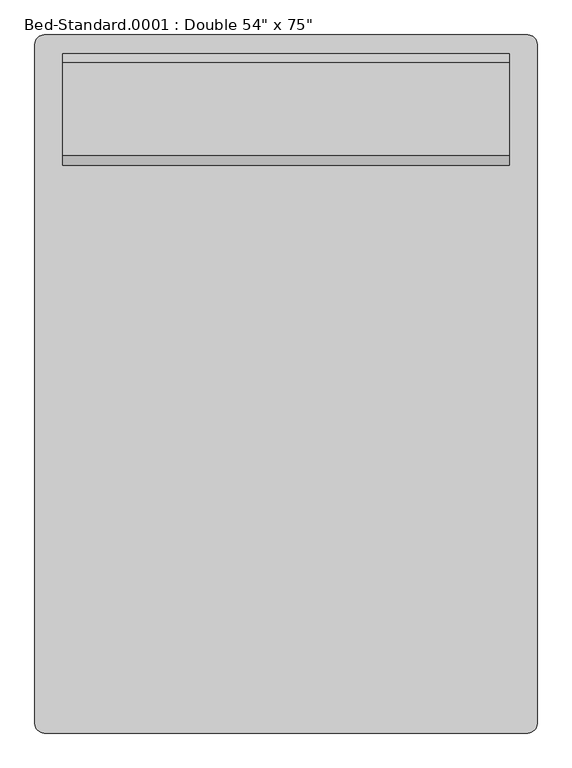
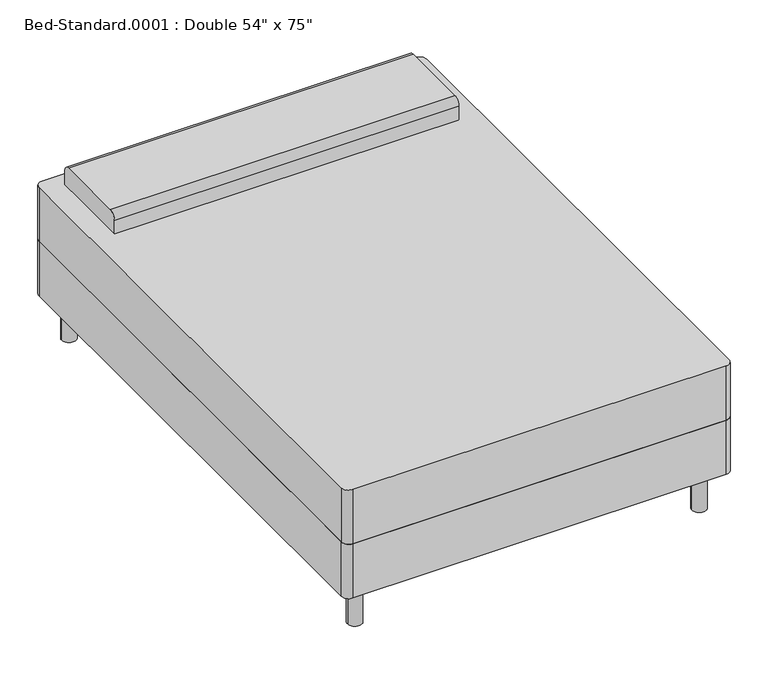
"""IFC4 building model written with IfcOpenShell, lengths in millimetres: furniture geometry."""

from ifc_helpers import new_model, si_unit, point, frame, frame_2d, origin, origin_with_axes, place, context, project, spatial, polyline, circle_curve, trimmed, segment, composite_curve, outline, extrude, source, transform, mapped, element, save


def furniture_0253826f(model_context):
    return source(origin(), model_context, "Body", "SweptSolid", [
        extrude(outline(composite_curve([segment(polyline([(-414.3114754, -972.695082), (-414.3114754, 881.504918)]), True, "CONTINUOUS"), segment(trimmed(circle_curve(frame_2d((-388.9114754, 881.504918)), 25.4), [point((-414.3114754, 881.504918))], [point((-388.9114754, 906.904918))], False, "CARTESIAN"), True, "CONTINUOUS"), segment(polyline([(-388.9114754, 906.904918), (931.8885246, 906.904918)]), True, "CONTINUOUS"), segment(trimmed(circle_curve(frame_2d((931.8885246, 881.504918)), 25.4), [point((931.8885246, 906.904918))], [point((957.2885246, 881.504918))], False, "CARTESIAN"), True, "CONTINUOUS"), segment(polyline([(957.2885246, 881.504918), (957.2885246, -972.695082)]), True, "CONTINUOUS"), segment(trimmed(circle_curve(frame_2d((931.8885246, -972.695082)), 25.4), [point((957.2885246, -972.695082))], [point((931.8885246, -998.095082))], False, "CARTESIAN"), True, "CONTINUOUS"), segment(polyline([(931.8885246, -998.095082), (-388.9114754, -998.095082)]), True, "CONTINUOUS"), segment(trimmed(circle_curve(frame_2d((-388.9114754, -972.695082)), 25.4), [point((-388.9114754, -998.095082))], [point((-414.3114754, -972.695082))], False, "CARTESIAN"), True, "CONTINUOUS")], self_intersect=False)), frame((0.0, 0.0, 152.4), z_axis=(0.0, 0.0, 1.0), x_axis=(1.0, 0.0, 0.0)), (0.0, 0.0, 1.0), 203.2),
        extrude(outline(composite_curve([segment(polyline([(551.304918, 558.8), (551.304918, 609.6)]), True, "CONTINUOUS"), segment(trimmed(circle_curve(frame_2d((576.704918, 609.6)), 25.4), [point((551.304918, 609.6))], [point((576.704918, 635.0))], False, "CARTESIAN"), True, "CONTINUOUS"), segment(polyline([(576.704918, 635.0), (830.704918, 635.0)]), True, "CONTINUOUS"), segment(trimmed(circle_curve(frame_2d((830.704918, 609.6)), 25.4), [point((830.704918, 635.0))], [point((856.104918, 609.6))], False, "CARTESIAN"), True, "CONTINUOUS"), segment(polyline([(856.104918, 609.6), (856.104918, 558.8), (551.304918, 558.8)]), True, "CONTINUOUS")], self_intersect=False)), frame((-338.1114754, 0.0, 0.0), z_axis=(1.0, 0.0, 0.0), x_axis=(0.0, 1.0, 0.0)), (0.0, 0.0, 1.0), 1219.2),
        extrude(outline(composite_curve([segment(trimmed(circle_curve(frame_2d((-338.1114754, 830.704918)), 25.4), [point((-363.5114754, 830.704918))], [point((-312.7114754, 830.704918))], False, "CARTESIAN"), True, "CONTINUOUS"), segment(trimmed(circle_curve(frame_2d((-338.1114754, 830.704918)), 25.4), [point((-312.7114754, 830.704918))], [point((-363.5114754, 830.704918))], False, "CARTESIAN"), True, "CONTINUOUS")], self_intersect=False)), origin_with_axes(), (0.0, 0.0, 1.0), 152.4),
        extrude(outline(composite_curve([segment(trimmed(circle_curve(frame_2d((881.0885246, 830.704918)), 25.4), [point((855.6885246, 830.704918))], [point((906.4885246, 830.704918))], False, "CARTESIAN"), True, "CONTINUOUS"), segment(trimmed(circle_curve(frame_2d((881.0885246, 830.704918)), 25.4), [point((906.4885246, 830.704918))], [point((855.6885246, 830.704918))], False, "CARTESIAN"), True, "CONTINUOUS")], self_intersect=False)), origin_with_axes(), (0.0, 0.0, 1.0), 152.4),
        extrude(outline(composite_curve([segment(trimmed(circle_curve(frame_2d((881.0885246, -921.895082)), 25.4), [point((855.6885246, -921.895082))], [point((906.4885246, -921.895082))], False, "CARTESIAN"), True, "CONTINUOUS"), segment(trimmed(circle_curve(frame_2d((881.0885246, -921.895082)), 25.4), [point((906.4885246, -921.895082))], [point((855.6885246, -921.895082))], False, "CARTESIAN"), True, "CONTINUOUS")], self_intersect=False)), origin_with_axes(), (0.0, 0.0, 1.0), 152.4),
        extrude(outline(composite_curve([segment(trimmed(circle_curve(frame_2d((-338.1114754, -921.895082)), 25.4), [point((-363.5114754, -921.895082))], [point((-312.7114754, -921.895082))], False, "CARTESIAN"), True, "CONTINUOUS"), segment(trimmed(circle_curve(frame_2d((-338.1114754, -921.895082)), 25.4), [point((-312.7114754, -921.895082))], [point((-363.5114754, -921.895082))], False, "CARTESIAN"), True, "CONTINUOUS")], self_intersect=False)), origin_with_axes(), (0.0, 0.0, 1.0), 152.4),
        extrude(outline(composite_curve([segment(polyline([(-388.9114754, 906.904918), (931.8885246, 906.904918)]), True, "CONTINUOUS"), segment(trimmed(circle_curve(frame_2d((931.8885246, 881.504918)), 25.4), [point((931.8885246, 906.904918))], [point((957.2885246, 881.504918))], False, "CARTESIAN"), True, "CONTINUOUS"), segment(polyline([(957.2885246, 881.504918), (957.2885246, -972.695082)]), True, "CONTINUOUS"), segment(trimmed(circle_curve(frame_2d((931.8885246, -972.695082)), 25.4), [point((957.2885246, -972.695082))], [point((931.8885246, -998.095082))], False, "CARTESIAN"), True, "CONTINUOUS"), segment(polyline([(931.8885246, -998.095082), (-388.9114754, -998.095082)]), True, "CONTINUOUS"), segment(trimmed(circle_curve(frame_2d((-388.9114754, -972.695082)), 25.4), [point((-388.9114754, -998.095082))], [point((-414.3114754, -972.695082))], False, "CARTESIAN"), True, "CONTINUOUS"), segment(polyline([(-414.3114754, -972.695082), (-414.3114754, 881.504918)]), True, "CONTINUOUS"), segment(trimmed(circle_curve(frame_2d((-388.9114754, 881.504918)), 25.4), [point((-414.3114754, 881.504918))], [point((-388.9114754, 906.904918))], False, "CARTESIAN"), True, "CONTINUOUS")], self_intersect=False)), frame((0.0, 0.0, 355.6), z_axis=(0.0, 0.0, 1.0), x_axis=(1.0, 0.0, 0.0)), (0.0, 0.0, 1.0), 203.2),
    ])


if __name__ == "__main__":
    model = new_model("IFC4")
    model_context = context("Model", 3, world=origin())
    ifc_project = project(units=[si_unit("LENGTHUNIT", "METRE", prefix="MILLI")], contexts=[model_context])
    site = spatial("IfcSite", under=ifc_project)
    building = spatial("IfcBuilding", under=site)
    placement = place(None, origin())
    furniture_shape = furniture_0253826f(model_context)
    element("IfcFurniture", 1, ObjectType="Bed-Standard.0001 : Double 54\" x 75\"", at=placement, inside=building, context=model_context, shape_type="MappedRepresentation", body=[
        mapped(furniture_shape, transform((0.0, 0.0, 0.0), x_axis=(1.0, 0.0, 0.0), y_axis=(0.0, 1.0, 0.0), z_axis=(0.0, 0.0, 1.0))),
    ])
    save(model, "model.ifc")

# Revit data of these elements
# Type "Bed-Standard.0001 : Double 54\" x 75\""
#   Assembly Code = "E2020200"
#   Length = 6' - 3"
#   Width = 4' - 6"
#   Leg Material = Steel, Chrome Plated
#   Mattress Material = Laminate, Linen, Matte
#   Default Elevation = 0
# Element 1 (IfcFurniture, "Bed-Standard.0001 : Double 54\" x 75\"")
#   Materials on its faces: "Linen, White", "Steel, Chrome Plated"
# Materials
#   "Steel, Chrome Plated": class "Metal", colour RGB 17 17 17, transparency 0, Description = "Chromiuim plated steel", Cost = 0
#   "Laminate, Linen, Matte": class "Plastic", colour RGB 249 239 230, transparency 0, Description = "Plastic Laminate - Linen, Matte", Cost = 0
#   "Linen, White": class "Textile", colour RGB 247 247 239, transparency 0, Description = "Linen, white", Cost = 0
